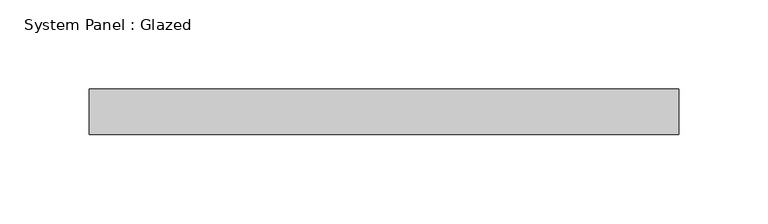
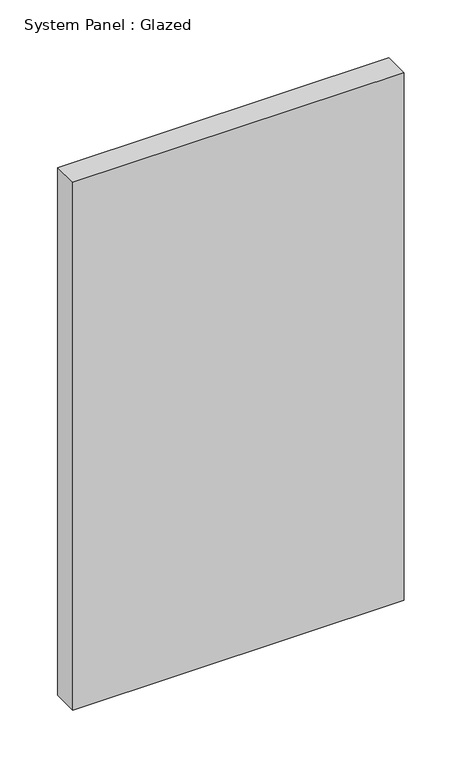
"""IFC4 building model written with IfcOpenShell, lengths in millimetres: plate geometry, System Panel : Glazed."""

from ifc_helpers import new_model, si_unit, origin, origin_with_axes, place, context, project, spatial, polyline, outline, extrude, source, transform, mapped, element, save


def system_panel_glazed_58f4fe82(model_context):
    return source(origin(), model_context, "Body", "SweptSolid", [
        extrude(outline(polyline([(165.1, 19.05), (-165.1, 19.05), (-165.1, 44.45), (165.1, 44.45), (165.1, 19.05)])), origin_with_axes(), (0.0, 0.0, 1.0), 555.8647026),
    ])


if __name__ == "__main__":
    model = new_model("IFC4")
    model_context = context("Model", 3, world=origin())
    ifc_project = project(units=[si_unit("LENGTHUNIT", "METRE", prefix="MILLI")], contexts=[model_context])
    site = spatial("IfcSite", under=ifc_project)
    building = spatial("IfcBuilding", under=site)
    placement = place(None, origin())
    system_panel_glazed_shape = system_panel_glazed_58f4fe82(model_context)
    element("IfcPlate", 1, ObjectType="System Panel : Glazed", at=placement, inside=building, context=model_context, shape_type="MappedRepresentation", body=[
        mapped(system_panel_glazed_shape, transform((0.0, 0.0, 0.0), x_axis=(1.0, 0.0, 0.0), y_axis=(0.0, 1.0, 0.0), z_axis=(0.0, 0.0, 1.0))),
    ])
    save(model, "model.ifc")

# Revit data of these elements
# Type "System Panel : Glazed"
#   Construction Type Id = "GSP4R"
#   Analytic Construction = "1/8 in Pilkington single glazing"
#   Visual Light Transmittance = 0.9
#   Solar Heat Gain Coefficient = 0.86
#   Heat Transfer Coefficient (U) = 1.18115 BTU/(h·ft²·°F)
#   Define Thermal Properties by = 1
# Element 1 (IfcPlate, "System Panel : Glazed")
#   Materials on its faces: "Glass"
# Materials
#   "Glass": class "Glass", colour RGB 0 128 192, transparency 0.75, Description = "Soda Lime Glass", Cost = 0
